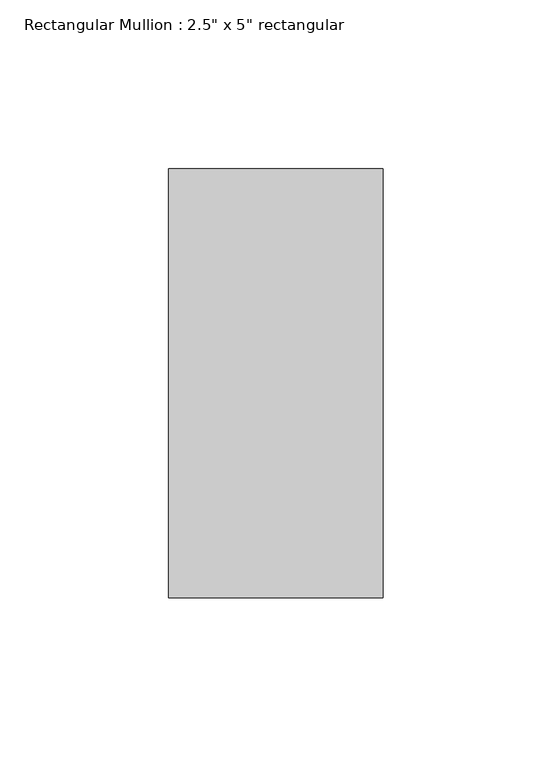
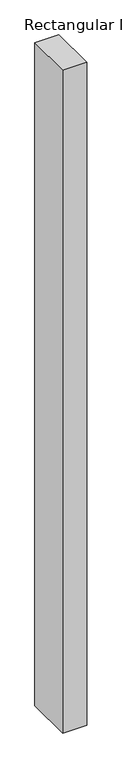
"""IFC4 building model written with IfcOpenShell, lengths in millimetres: member geometry."""

from ifc_helpers import new_model, si_unit, frame, origin, place, context, project, spatial, polyline, outline, extrude, source, transform, mapped, element, save


def member_3ffc8328(model_context):
    return source(origin(), model_context, "Body", "SweptSolid", [
        extrude(outline(polyline([(0.0, 63.5), (0.0, -63.5), (-63.5, -63.5), (-63.5, 63.5), (0.0, 63.5)])), frame((0.0, 0.0, -1849.9041833), z_axis=(0.0, 0.0, 1.0), x_axis=(1.0, 0.0, 0.0)), (0.0, 0.0, 1.0), 1849.9041833),
    ])


if __name__ == "__main__":
    model = new_model("IFC4")
    model_context = context("Model", 3, world=origin())
    ifc_project = project(units=[si_unit("LENGTHUNIT", "METRE", prefix="MILLI")], contexts=[model_context])
    site = spatial("IfcSite", under=ifc_project)
    building = spatial("IfcBuilding", under=site)
    placement = place(None, origin())
    member_shape = member_3ffc8328(model_context)
    element("IfcMember", 1, ObjectType="Rectangular Mullion : 2.5\" x 5\" rectangular", at=placement, inside=building, context=model_context, shape_type="MappedRepresentation", body=[
        mapped(member_shape, transform((0.0, 0.0, 0.0), x_axis=(1.0, 0.0, 0.0), y_axis=(0.0, 1.0, 0.0), z_axis=(0.0, 0.0, 1.0))),
    ])
    save(model, "model.ifc")

# Revit data of these elements
# Type "Rectangular Mullion : 2.5\" x 5\" rectangular"
#   built-in parameter 1007304 = 0.416667 (stored number, unit not read)
#   built-in parameter 1007301 = 0.104167 (stored number, unit not read)
#   built-in parameter 1007300 = 0.104167 (stored number, unit not read)
# Element 1 (IfcMember, "Rectangular Mullion : 2.5\" x 5\" rectangular")
#   Materials on its faces: "Aluminum"
# Materials
#   "Aluminum": class "Metal", colour RGB 247 247 247, transparency 0, Description = "Aluminum 6061", Cost = 0
